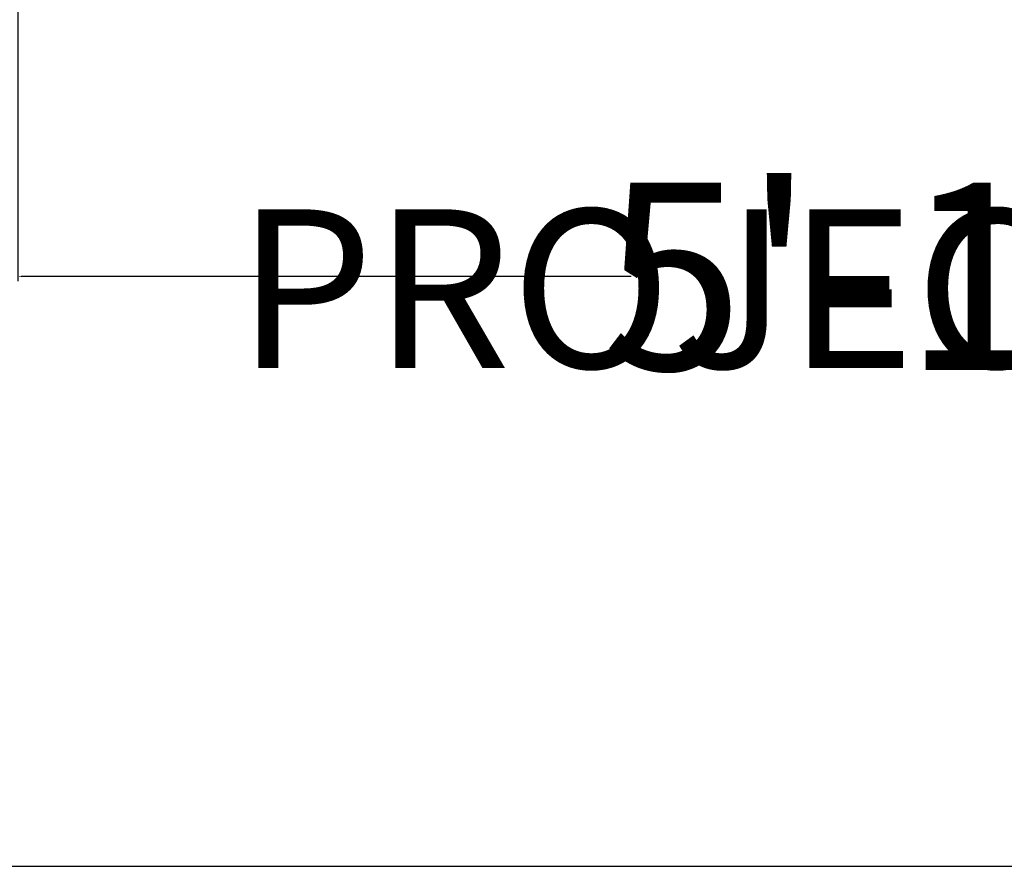
# Model space of a CAD drawing. Units: inches. Extents: x 0 to 4258, y 0 to 3769.
# Tile 4 of 30: x 3726 to 3762, y 2939 to 2971. Entities that reach past the tile are written whole.
import ezdxf

# ---------------------------------------------------------------- set-up
doc = ezdxf.new("R2010")
doc.units = ezdxf.units.IN
doc.header["$MEASUREMENT"] = 0
for name, color, linetype, lineweight in [('A-ANNO-DIMS', 250, 'Continuous', 18), ('A-ANNO-TEXT', 250, 'Continuous', 18), ('C-PROP', 150, 'Continuous', 25)]:
    doc.layers.add(name, color=color, linetype=linetype, lineweight=lineweight)
doc.styles.get("Standard").update_dxf_attribs({"font": 'arial.ttf'})
doc.dimstyles.get("Standard").update_dxf_attribs({"dimtxt": 7, "dimasz": 0.18, "dimexe": 0.18, "dimexo": 0.0625, "dimgap": 0.09, "dimtad": 0, "dimtih": 1, "dimtoh": 1, "dimzin": 0, "dimdsep": 46, "dimlunit": 3, "dimtxsty": 'Standard', "dimcen": 0.09, "dimadec": 0, "dimazin": 0, "dimtfac": 1, "dimtofl": 0, "dimtmove": 0, "dimatfit": 3, "dimfxl": 1, "dimtolj": 1, "dimtzin": 0, "dimarcsym": 0})

# ---------------------------------------------------------------- blocks, each defined once
blk = doc.blocks.new('*D67')
at = {"layer": 'A-ANNO-DIMS', "color": 0, "lineweight": -2, "transparency": 16777216}
for p, q in [((3725.58, 2982.693), (3725.58, 2961.112)), ((3795.713, 2982.693), (3795.713, 2961.112)), ((3725.76, 2961.292), (3748.533, 2961.292)), ((3795.533, 2961.292), (3772.76, 2961.292))]:
    blk.add_line(p, q, dxfattribs=at)
at = {"layer": 'A-ANNO-DIMS', "color": 0, "transparency": 16777216}
for points in [[(3725.76, 2961.322), (3725.76, 2961.262), (3725.58, 2961.292)], [(3795.533, 2961.322), (3795.533, 2961.262), (3795.713, 2961.292)]]:
    blk.add_solid(points, dxfattribs=at)
at = {"layer": 'Defpoints', "color": 0, "transparency": 16777216}
for p in [(3725.58, 2982.755), (3795.713, 2982.755), (3795.713, 2961.292)]:
    blk.add_point(p, dxfattribs=at)
at = {"layer": 'A-ANNO-DIMS', "color": 0, "transparency": 16777216, "insert": (3760.646, 2961.292), "char_height": 7, "attachment_point": 5}
blk.add_mtext('\\A1;5\'-10"', dxfattribs=at)

msp = doc.modelspace()

# ---------------------------------------------------------------- linework, layer by layer
at = {"layer": 'C-PROP'}
msp.add_line((3683.892, 2939.211), (3766.077, 2939.211), dxfattribs=at)

# ---------------------------------------------------------------- texts
at = {"layer": 'A-ANNO-TEXT'}
msp.add_text('PROJECTION', height=5.939, dxfattribs=at).set_placement((3733.76, 2957.861))

# ---------------------------------------------------------------- dimensions: what is measured, and where the dimension line sits
at = {"layer": 'A-ANNO-DIMS'}
dim = msp.add_linear_dim(base=(3795.713, 2961.292), p1=(3725.58, 2982.755), p2=(3795.713, 2982.755), dimstyle='Standard', override={"dimdec": 1, "dimlfac": 1, "dimrnd": 0, "dimzin": 1, "dimdsep": 46, "dimlunit": 4, "dimfrac": 2}, dxfattribs=at)
dim.commit()
dim.dimension.update_dxf_attribs({"geometry": '*D67', "text_midpoint": (3760.646, 2961.292)})

doc.saveas('drawing.dxf')
